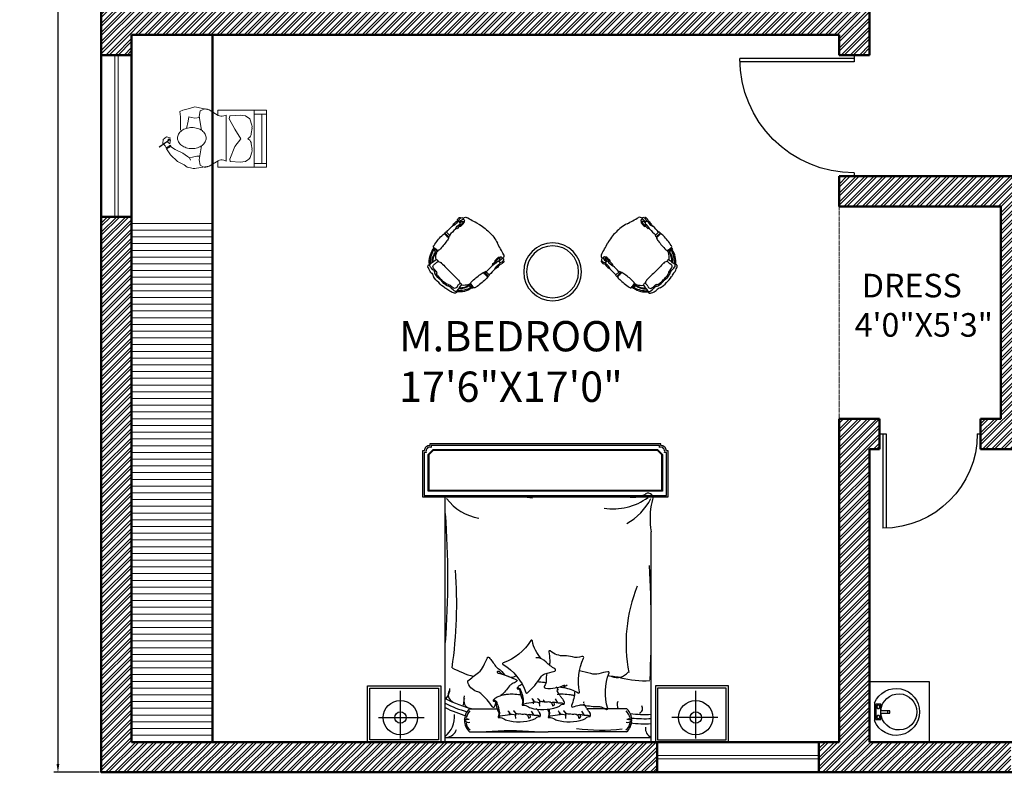
# Model space of a CAD drawing. Units: inches. Extents: x 3590 to 5167, y 65 to 1917.
# Tile 26 of 100: x 4396 to 4688, y 1326 to 1549. Entities that reach past the tile are written whole.
import ezdxf

# ---------------------------------------------------------------- set-up
doc = ezdxf.new("R2010")
doc.units = ezdxf.units.IN
doc.linetypes.add('DASHED', pattern=[0.75, 0.5, -0.25])
for name, color, linetype, lineweight in [('A-ANNO-DIMS', 2, 'Continuous', 18), ('A-AREA-IDEN', 7, 'Continuous', 18), ('A-DOOR', 3, 'Continuous', 25), ('A-FLOR-FIXT', 8, 'Continuous', 18), ('A-FURN', 21, 'Continuous', 18), ('A-GLAZ', 4, 'Continuous', 18), ('A-WALL', 7, 'Continuous', 50), ('A-WALL-PATT', 251, 'Continuous', 13), ('S-BEAM-OVHD', 7, 'DASHED', 18)]:
    doc.layers.add(name, color=color, linetype=linetype, lineweight=lineweight)
for name, color, linetype in [('FUR', 42, 'Continuous'), ('furn', 7, 'Continuous'), ('HA-FUR', 8, 'Continuous'), ('HA-P', 8, 'Continuous'), ('SAN', 5, 'Continuous'), ('SANTEH', 7, 'Continuous'), ('wood', 26, 'Continuous')]:
    doc.layers.add(name, color=color, linetype=linetype)
doc.styles.get("Standard").update_dxf_attribs({"font": 'arial.ttf'})
doc.dimstyles.new('ISO-25', dxfattribs={"dimtxt": 9, "dimasz": 2.5, "dimexe": 1.25, "dimexo": 0.625, "dimtad": 1, "dimdec": 1, "dimlunit": 3, "dimtxsty": 'Standard', "dimcen": 2.5, "dimadec": 0, "dimazin": 0, "dimtfac": 1, "dimtdec": 1, "dimtmove": 0, "dimatfit": 3, "dimfxl": 1, "dimarcsym": 0})

# ---------------------------------------------------------------- blocks, each defined once
blk = doc.blocks.new('*D102')
at = {"layer": 'A-ANNO-DIMS', "color": 0, "lineweight": -2, "transparency": 16777216}
for p, q in [((4419.65, 1806), (4406.15, 1806)), ((4407.4, 1803.5), (4407.4, 1328.5)), ((4419.65, 1326), (4406.15, 1326))]:
    blk.add_line(p, q, dxfattribs=at)
at = {"layer": 'A-ANNO-DIMS', "color": 0, "transparency": 16777216}
for points in [[(4406.98, 1803.5), (4407.82, 1803.5), (4407.4, 1806)], [(4406.98, 1328.5), (4407.82, 1328.5), (4407.4, 1326)]]:
    blk.add_solid(points, dxfattribs=at)
at = {"layer": 'Defpoints', "color": 0, "transparency": 16777216}
for p in [(4420.27, 1806), (4407.4, 1326), (4420.27, 1326)]:
    blk.add_point(p, dxfattribs=at)
at = {"layer": 'A-ANNO-DIMS', "color": 0, "transparency": 16777216, "insert": (4402.18, 1566), "char_height": 9, "attachment_point": 5, "rotation": 90}
blk.add_mtext("40'", dxfattribs=at)
blk = doc.blocks.new('D2')
for p, q in [((1, 0), (1, 28)), ((2, 0), (2, 27.98)), ((0, 0), (2, 0)), ((29, 0), (30, 0))]:
    blk.add_line(p, q)
at = {"ltscale": 0.5}
blk.add_arc((1, 0), 28, 0, 90, dxfattribs=at)
blk = doc.blocks.new('D1')
for p, q in [((1, 0), (1, 34)), ((2, 0), (2, 33.99)), ((0, 0), (2, 0)), ((35, 0), (36, 0))]:
    blk.add_line(p, q)
at = {"ltscale": 0.5}
blk.add_arc((1, 0), 34, 0, 90, dxfattribs=at)
blk = doc.blocks.new('r11')
at = {"layer": 'SANTEH', "ltscale": 5}
for p, q in [((0, 0), (600, 0)), ((0, -600), (0, 0)), ((600, 0), (600, -600)), ((210.5, -50), (389.5, -50)), ((210.5, -50), (210.5, -50)), ((223.8, -63.2), (376.2, -63.2)), ((223.8, -113.2), (223.8, -63.2)), ((232.7, -78.7), (249.2, -69.1)), ((232.7, -97.7), (232.7, -78.7)), ((249.2, -107.2), (232.7, -97.7)), ((249.2, -69.1), (265.7, -78.7)), ((265.7, -97.7), (249.2, -107.2)), ((265.7, -78.7), (265.7, -97.7)), ((334.3, -78.7), (350.8, -69.1)), ((334.3, -97.7), (334.3, -78.7)), ((350.8, -107.2), (334.3, -97.7)), ((350.8, -69.1), (367.3, -78.7)), ((367.3, -97.7), (350.8, -107.2)), ((367.3, -78.7), (367.3, -97.7)), ((376.2, -63.2), (376.2, -113.2)), ((376.2, -113.2), (223.8, -113.2)), ((288, -201.6), (288, -113.2)), ((312, -184.3), (288, -184.3)), ((312, -113.2), (312, -201.6)), ((312, -201.6), (288, -201.6)), ((600, -600), (0, -600))]:
    blk.add_line(p, q, dxfattribs=at)
for centre, radius, start, end in [((300, -266.2), 234, 112.50001, 67.49999), ((300, -293), 180.2, 93.8183, 86.1817)]:
    blk.add_arc(centre, radius, start, end, dxfattribs=at)
blk = doc.blocks.new('A$C0A42580C')
at = {"layer": 'SAN'}
for p, q in [((0.2873, 0.0301), (0.2873, 0.4484)), ((2.8678, 0.0301), (2.8678, 0.4484)), ((0.0949, 0.2135), (0.4958, 0.2135)), ((3.0601, 0.2135), (2.6592, 0.2135))]:
    blk.add_line(p, q, dxfattribs=at)
for centre, radius in [((0.2873, 0.2135), 0.15), ((2.8678, 0.2135), 0.15), ((0.2873, 0.2135), 0.05), ((2.8678, 0.2135), 0.05)]:
    blk.add_circle(centre, radius, dxfattribs=at)
at = {"layer": 'wood'}
for p, q in [((0.6775, 0.8851), (0.6775, 2.1392)), ((2.4775, 0.8016), (2.4775, 1.838)), ((2.4775, 0), (2.4775, 0.8016)), ((1.6633, 0.3438), (1.6434, 0.3761)), ((0.888, 0.289), (1.1327, 0.289)), ((1.4538, 0.2362), (1.434, 0.2685)), ((1.5, 0.3423), (1.5016, 0.3142)), ((1.8919, 0.2362), (1.8721, 0.2685)), ((2.267, 0.289), (1.9163, 0.289)), ((1.2906, 0.2348), (1.2921, 0.2067)), ((1.7287, 0.2348), (1.7302, 0.2067)), ((0.8909, 0.089), (1.5775, 0.089)), ((2.2642, 0.089), (1.5775, 0.089)), ((0.6775, 0.039), (2.4775, 0.039)), ((0.6775, 0), (2.4775, 0))]:
    blk.add_line(p, q, dxfattribs=at)
blk.add_lwpolyline([(0.6775, 0), (0.6775, 0.8851)], dxfattribs=at)
for points in [[(1.516, 0.7294, -0.128392), (1.4401, 0.8834, 0.70791), (1.427, 0.8863, -0.16964), (1.1848, 0.6919, 0.664036), (1.184, 0.6776, -0.184649), (1.3819, 0.4332, 0.662242), (1.3969, 0.4309, 0.078539), (1.5137, 0.5669, -0.1736), (1.5484, 0.5947, -0.02159), (1.6357, 0.6205, 0.697276), (1.6379, 0.6405, -0.093019), (1.5606, 0.699, 0.216632), (1.4719, 0.7371, -2.511293)], [(1.6795, 0.4818, 0.263265), (1.7191, 0.4839, -0.026108), (1.743, 0.4973, 0.027613), (1.7137, 0.4764, -0.089259), (1.8403, 0.429, 0.662242), (1.8528, 0.4376, -0.162037), (1.8882, 0.732, 0.676499), (1.8733, 0.748, -0.160513), (1.7901, 0.7439, 0.07473), (1.7202, 0.7523, -0.187721), (1.5966, 0.7963, 0.70791), (1.5851, 0.7895, -0.010003), (1.5921, 0.7143, -0.07079), (1.5891, 0.6719, 0.099539)], [(1.1211, 0.3454, 0.032543), (1.1095, 0.3091, -0.658965), (1.0917, 0.3063, 0.074753), (0.9887, 0.4234, 0.100988), (0.953, 0.4429, -0.270711), (0.8753, 0.5273, -0.276825), (0.8775, 0.5337, -0.014937), (0.9701, 0.6081, 0.134834), (1.0135, 0.6643, -0.023706), (1.0474, 0.7372, -0.664036), (1.0616, 0.7394, -0.035987), (1.119, 0.6627, 0.118631), (1.1415, 0.6412, -0.132738), (1.1955, 0.5864)], [(1.1759, 0.5928, 0.013884), (1.1549, 0.6131, 0.174178), (1.1437, 0.6177, 0.104076), (1.1358, 0.6165, 0.389829), (1.1324, 0.6097, 0.296089), (1.1415, 0.6019, -0.036701), (1.1572, 0.5985, -0.040547), (1.3022, 0.543, -0.70791), (1.3021, 0.5296, -0.016811), (1.2631, 0.5085, 0.11866), (1.2414, 0.4904, -0.048791), (1.1649, 0.4055, 0.103757)], [(1.8113, 0.4446, -0.069098), (1.7831, 0.3187, 0.658965), (1.7961, 0.3062, -0.049789), (1.8516, 0.3234, -0.103757), (1.8905, 0.3233, 0.055725), (2.0203, 0.3103, -0.11866), (2.0478, 0.304, 0.016811), (2.0881, 0.2856, 0.70791), (2.0989, 0.2936, -0.16964), (2.1104, 0.604, 0.664036), (2.1001, 0.6139, 0.023706), (2.0214, 0.597, -0.134834), (1.9505, 0.5976, 0.012748), (1.8522, 0.6228)], [(1.5674, 0.601, 0.057807), (1.5606, 0.5339, -0.173425), (1.5457, 0.49, 0.589988), (1.5538, 0.4706, 0.137312), (1.7236, 0.4985, 0.137312)], [(1.3107, 0.4764, 0.145733), (1.3069, 0.4677, 0.488583), (1.3089, 0.4657, -0.012138), (1.3131, 0.4661, -0.125673), (1.3213, 0.4646, -0.750706)], [(1.3153, 0.4751, -0.274893), (1.3379, 0.4529, 0.051436), (1.3468, 0.4293, -0.086628), (1.3532, 0.4078, 0.040196), (1.3593, 0.3772, -0.184744), (1.3556, 0.3344, -2.554464)], [(1.317, 0.4683, -0.060098), (1.3283, 0.4571, -0.16247), (1.3313, 0.4487, 0.120018), (1.3493, 0.3815, -0.060072), (1.3541, 0.3695, -0.13107), (1.3541, 0.3395, -0.024415), (1.3534, 0.3373, 0.070398), (1.3503, 0.3233, 0.528689), (1.3524, 0.3216, -0.069388), (1.3557, 0.3222, -0.158233), (1.4075, 0.3065, 0.085461), (1.4255, 0.2981, 0.147196), (1.6571, 0.3041, 0.10985), (1.6823, 0.3191, -0.179095), (1.7126, 0.3319, -2.318897)], [(1.1013, 0.3688, 0.145733), (1.0975, 0.3601, 0.488583), (1.0995, 0.3581, -0.012138), (1.1036, 0.3585, -0.125673), (1.1119, 0.357, -0.750706)], [(1.1059, 0.3675, -0.274893), (1.1285, 0.3453, 0.051436), (1.1373, 0.3217, -0.086628), (1.1438, 0.3003, 0.040196), (1.1499, 0.2696, -0.184744), (1.1462, 0.2269, -2.554464)], [(1.1076, 0.3607, -0.060098), (1.1189, 0.3495, -0.16247), (1.1219, 0.3411, 0.120018), (1.1399, 0.2739, -0.060072), (1.1447, 0.2619, -0.13107), (1.1447, 0.2319, -0.024415), (1.144, 0.2297, 0.070398), (1.1409, 0.2157, 0.528689), (1.143, 0.2141, -0.069388), (1.1463, 0.2146, -0.158233), (1.1981, 0.1989, 0.085461), (1.2161, 0.1905, 0.147196), (1.4477, 0.1965, 0.10985), (1.4728, 0.2115, -0.179095), (1.5032, 0.2244, -2.318897)], [(1.3509, 0.3219, -0.117141), (1.3688, 0.335, -0.025084), (1.4533, 0.348, 0.033691)], [(1.4359, 0.3803, -0.198519), (1.452, 0.3494, 0.826402), (1.4558, 0.349, 0.095956), (1.4561, 0.3528, 0.242899), (1.4461, 0.3686, -17.523452)], [(1.5447, 0.3525, -0.083557), (1.507, 0.3546, 0.203162), (1.4851, 0.3792, -0.208037), (1.5043, 0.3409, 0.124669), (1.4432, 0.3469, 0.965934)], [(1.5394, 0.3688, 0.145733), (1.5356, 0.3601, 0.488583), (1.5376, 0.3581, -0.012138), (1.5418, 0.3585, -0.125673), (1.55, 0.357, -0.750706)], [(1.5447, 0.3525, -0.008229), (1.5728, 0.3519, 0.033691)], [(1.5728, 0.3519, -0.46905), (1.6152, 0.321, 0.420988), (1.62, 0.3169, 0.857652), (1.6221, 0.3484, 0.548526)], [(1.603, 0.3451, -0.099719), (1.6221, 0.3484, 0.102691)], [(1.6214, 0.3487, -0.010168), (1.6558, 0.3447, 0.033691), (1.6907, 0.3423, -0.220869), (1.7148, 0.3311, -0.288972)], [(1.2265, 0.2728, -0.198519), (1.2426, 0.2418, 0.826402), (1.2463, 0.2415, 0.095956), (1.2467, 0.2452, 0.242899), (1.2366, 0.2611, -17.523452)], [(1.3353, 0.2449, -0.083557), (1.2976, 0.247, 0.203162), (1.2757, 0.2717, -0.208037), (1.2948, 0.2333, 0.124669), (1.2338, 0.2393, 0.965934)], [(1.5721, 0.286, 0.022869), (1.578, 0.2739, -0.060072), (1.5828, 0.2619, -0.13107), (1.5828, 0.2319, -0.024415), (1.5821, 0.2297, 0.070398), (1.579, 0.2157, 0.528689), (1.5811, 0.2141, -0.069388), (1.5844, 0.2146, -0.158233), (1.6362, 0.1989, 0.085461), (1.6542, 0.1905, 0.147196), (1.8858, 0.1965, 0.10985), (1.911, 0.2115, -0.179095), (1.9413, 0.2244, -2.318897)], [(1.5838, 0.2873, 0.023398), (1.588, 0.2696, -0.184744), (1.5843, 0.2269, -2.554464)], [(1.6646, 0.2728, -0.198519), (1.6807, 0.2418, 0.826402), (1.6845, 0.2415, 0.095956), (1.6848, 0.2452, 0.242899), (1.6748, 0.2611, -17.523452)], [(1.7734, 0.2449, -0.083557), (1.7357, 0.247, 0.203162), (1.7138, 0.2717, -0.208037), (1.733, 0.2333, 0.124669), (1.6719, 0.2393, 0.965934)], [(1.1415, 0.2143, -0.117141), (1.1594, 0.2274, -0.025084), (1.2439, 0.2405, 0.033691)], [(1.3353, 0.2449, -0.008229), (1.3633, 0.2443, 0.033691)], [(1.3633, 0.2443, -0.46905), (1.4058, 0.2134, 0.420988), (1.4106, 0.2093, 0.857652), (1.4127, 0.2408, 0.548526)], [(1.3936, 0.2375, -0.099719), (1.4127, 0.2408, 0.102691)], [(1.412, 0.2411, -0.010168), (1.4464, 0.2371, 0.033691), (1.4812, 0.2348, -0.220869), (1.5054, 0.2235, -0.288972)], [(1.5796, 0.2143, -0.117141), (1.5975, 0.2274, -0.025084), (1.682, 0.2405, 0.033691)], [(1.7734, 0.2449, -0.008229), (1.8015, 0.2443, 0.033691)], [(1.8015, 0.2443, -0.46905), (1.8439, 0.2134, 0.420988), (1.8487, 0.2093, 0.857652), (1.8508, 0.2408, 0.548526)], [(1.8317, 0.2375, -0.099719), (1.8508, 0.2408, 0.102691)], [(1.8501, 0.2411, -0.010168), (1.8845, 0.2371, 0.033691), (1.9193, 0.2348, -0.220869), (1.9435, 0.2235, -0.288972)]]:
    blk.add_lwpolyline(points, format="xyb", dxfattribs=at)
for points in [[(0.64, 0), (0, 0), (0, 0.49), (0.64, 0.49)], [(0.62, 0.02), (0.02, 0.02), (0.02, 0.47), (0.62, 0.47)], [(2.515, 0), (3.155, 0), (3.155, 0.49), (2.515, 0.49)], [(2.535, 0.02), (3.135, 0.02), (3.135, 0.47), (2.535, 0.47)]]:
    blk.add_lwpolyline(points, close=True, dxfattribs=at)
for centre, radius, start, end in [((1.0344, -2.14), 4.292, 84.56078, 94.7164), ((2.3125, 2.3833), 0.2443, 254.1515, 300.95574), ((2.4501, 2.1309), 0.0445, 324.18954, 118.92203), ((1.0494, 2.4026), 0.4515, 217.47941, 260.35986), ((2.0208, -11.0786), 13.2288, 88.75549, 92.51133), ((2.1491, 2.5471), 0.5083, 260.65485, 306.44155), ((2.0168, 2.3573), 0.5127, 299.08175, 333.44367), ((3.1371, 1.9502), 0.669, 166.6404, 189.65708), ((-7.0839, 1.4328), 7.7858, 355.84817, 4.15183), ((-3.167, 1.2143), 3.9465, 351.77286, 4.18386), ((-7.2439, 0.9937), 9.7233, 357.34474, 3.23068), ((3.5803, 0.8622), 1.3213, 157.81295, 191.15154), ((1.1611, 1.4181), 0.8768, 241.21362, 254.41879), ((2.181, 0.6859), 0.1221, 247.37754, 321.13165), ((1.2583, 0.6364), 0.0695, 238.58923, 301.92671), ((1.4714, 0.0722), 0.4528, 80.62397, 88.74059), ((1.4035, -0.3388), 0.8693, 79.71489, 80.62397), ((1.7861, -2.1601), 2.7557, 80.89877, 83.46656), ((2.4192, 1.3819), 0.8461, 255.77539, 273.25587), ((0.5904, 0.4689), 0.13, 317.38218, 359.70393), ((0.7723, 0.4131), 0.0674, 147.68233, 245.79865), ((1.3546, 0.4469), 0.0529, 114.21284, 146.15395), ((2.6126, -2.3504), 3.1201, 113.83178, 114.21284), ((1.6301, 0.4539), 0.0342, 31.14095, 54.95422), ((1.6709, 0.4489), 0.0156, 131.9623, 212.08127), ((1.6729, 0.4422), 0.0178, 140.41793, 157.63267), ((1.7235, 0.4818), 0.0777, 212.08127, 227.364), ((1.6635, 0.4499), 0.00568, 95.52245, 140.41793), ((1.5664, 0.4154), 0.1086, 24.20989, 31.14095), ((1.6627, 0.4587), 0.00309, 275.52245, 24.20989), ((1.1611, 1.3191), 1.0568, 242.76671, 257.10398), ((0.0312, 0.4583), 0.8174, 350.42368, 356.2506), ((0.9021, 0.3562), 0.0605, 155.8342, 254.41058), ((1.1452, 0.3394), 0.0529, 114.21284, 146.15395), ((2.4032, -2.458), 3.1201, 113.55686, 114.21284), ((1.2046, 0.2912), 0.121, 99.42032, 113.55686), ((1.2774, -0.1478), 0.5659, 95.90379, 99.42032), ((1.2626, -0.005), 0.4223, 88.74059, 95.90379), ((1.2619, -0.0354), 0.4528, 80.62397, 88.74059), ((1.1941, -0.4464), 0.8693, 79.45871, 80.62397), ((1.4207, 0.3463), 0.0342, 31.14095, 54.95422), ((1.4614, 0.3413), 0.0156, 131.9623, 212.08127), ((1.4635, 0.3347), 0.0178, 140.41793, 157.63267), ((1.4541, 0.3424), 0.00568, 95.52245, 140.41793), ((1.357, 0.3078), 0.1086, 24.20989, 31.14095), ((1.4533, 0.3511), 0.00309, 275.52245, 24.20989), ((1.7007, -0.005), 0.4223, 88.74059, 95.90379), ((1.6391, 0.3902), 0.0469, 17.32618, 47.364), ((1.7106, 0.4125), 0.028, 197.32618, 226.17302), ((1.6431, 0.3422), 0.0695, 26.61764, 46.17302), ((1.8202, 0.431), 0.1287, 206.61764, 215.96192), ((1.7001, -0.0354), 0.4528, 80.62397, 88.74059), ((1.6975, 0.3419), 0.023, 350.76434, 35.96192), ((1.6322, -0.4464), 0.8693, 78.43923, 80.62397), ((1.9016, 0.3347), 0.0178, 140.41793, 157.63267), ((1.8922, 0.3424), 0.00568, 95.52245, 140.41793), ((2.2511, 0.3256), 0.071, 155.86842, 211.04513), ((1.1611, 1.3191), 1.0937, 243.75553, 254.4906), ((1.1611, 1.2816), 1.0937, 243.75553, 254.38927), ((0.9846, 0.1903), 0.1381, 134.39284, 227.23745), ((0.9986, 0.1735), 0.1427, 136.58239, 164.9725), ((1.5012, 0.305), 0.028, 197.32618, 226.17302), ((1.4337, 0.2347), 0.0695, 26.61764, 46.17302), ((1.6108, 0.3235), 0.1287, 206.61764, 215.96192), ((1.715, 0.3349), 0.00379, 207.1817, 328.02977), ((1.7058, 0.3406), 0.0145, 328.02977, 350.76434), ((1.9522, 0.3743), 0.0777, 212.08127, 227.364), ((1.8678, 0.2827), 0.0469, 17.32618, 47.364), ((1.9393, 0.305), 0.028, 197.32618, 226.17302), ((1.8718, 0.2347), 0.0695, 26.61764, 46.17302), ((2.0489, 0.3235), 0.1287, 206.61764, 215.96192), ((2.1565, 0.1735), 0.1427, 15.0275, 43.41761), ((2.1704, 0.1903), 0.1381, 312.76255, 45.60716), ((2.3616, 0.2915), 0.0419, 290.78583, 35.36309), ((0.5293, 0.2241), 0.2307, 309.63048, 4.27465), ((0.8396, 0.185), 0.0112, 314.89662, 45.10338), ((0.8413, 0.1846), 0.0128, 299.47062, 57.44416), ((0.8844, 0.2286), 0.0569, 229.70587, 281.11527), ((0.8802, 0.1371), 0.0592, 81.47786, 123.11925), ((0.8698, 0.1793), 0.0229, 77.14902, 159.1786), ((1.5055, 0.2273), 0.00379, 207.1817, 328.02977), ((1.4881, 0.2344), 0.023, 350.76434, 35.96192), ((1.4964, 0.233), 0.0145, 328.02977, 350.76434), ((1.9436, 0.2273), 0.00379, 207.1817, 328.02977), ((1.9262, 0.2344), 0.023, 350.76434, 35.96192), ((1.9345, 0.233), 0.0145, 328.02977, 350.76434), ((2.2706, 0.2286), 0.0569, 258.88473, 310.29413), ((2.2749, 0.1371), 0.0592, 56.88075, 98.52214), ((2.2853, 0.1793), 0.0229, 20.8214, 102.85098), ((2.4192, 1.2667), 1.0261, 263.09035, 273.25587), ((2.3138, 0.1846), 0.0128, 122.55584, 240.52938), ((2.3154, 0.185), 0.0112, 134.89662, 225.10338), ((2.4192, 1.2667), 1.0629, 263.94374, 273.25587), ((0.6729, 0.151), 0.1135, 279.23824, 338.73819), ((0.9466, 0.1765), 0.0862, 185.53723, 234.68694), ((1.2481, -2.5919), 2.6893, 85.4722, 94.5278), ((2.0447, 1.7022), 1.5979, 262.13639, 276.48786), ((2.2085, 0.1765), 0.0862, 305.31306, 354.46277), ((2.4192, 1.2218), 1.0629, 263.23622, 273.25587), ((2.508, 0.1152), 0.0792, 169.94668, 248.24015)]:
    blk.add_arc(centre, radius, start, end, dxfattribs=at)
blk = doc.blocks.new('A$C623F1DA0')
at = {"layer": 'FUR'}
blk.add_lwpolyline([(0.628, 2.912, 0.414214), (0.562, 2.978), (0.562, 3), (0, 3), (0, 0), (0.562, 0), (0.562, 0.022, 0.414214), (0.628, 0.088), (0.65, 0.088), (0.65, 2.912)], format="xyb", close=True, dxfattribs=at)
at = {"layer": 'HA-FUR'}
blk.add_lwpolyline([(0.603, 2.892, 0.710288), (0.542, 2.953), (0.542, 2.98), (0.02, 2.98), (0.02, 0.02), (0.542, 0.02), (0.542, 0.047, 0.710288), (0.603, 0.108), (0.63, 0.108), (0.63, 2.892)], format="xyb", close=True, dxfattribs=at)
at = {"layer": 'HA-P'}
for points in [[(0.07, 2.93), (0.521, 2.93), (0.58, 2.871), (0.58, 0.129), (0.521, 0.07), (0.07, 0.07)], [(0.08, 2.92), (0.517, 2.92), (0.57, 2.867), (0.57, 0.133), (0.517, 0.08), (0.08, 0.08)]]:
    blk.add_lwpolyline(points, close=True, dxfattribs=at)
blk = doc.blocks.new('CHAIR6')
at = {"layer": 'furn'}
for p, q in [((0.41, 0.26), (0.409, 0.318)), ((0.428, 0.318), (0.427, 0.263)), ((0.41, -0.26), (0.409, -0.318)), ((0.428, -0.318), (0.427, -0.263))]:
    blk.add_line(p, q, dxfattribs=at)
for centre in [(0.405, 0.315), (0.405, 0.306), (0.217, 0.287), (0.219, 0.277), (0.22, 0.268), (0.221, 0.26), (0.222, 0.252), (0.223, 0.243), (0.405, 0.298), (0.405, 0.29), (0.406, 0.281), (0.405, 0.273), (0.406, 0.264), (0.217, -0.287), (0.219, -0.277), (0.22, -0.268), (0.221, -0.26), (0.222, -0.252), (0.223, -0.243), (0.406, -0.264), (0.405, -0.273), (0.406, -0.281), (0.405, -0.29), (0.405, -0.298), (0.405, -0.306), (0.405, -0.315)]:
    blk.add_circle(centre, 0.00425, dxfattribs=at)
for centre, radius, start, end in [((0.237, 0.291), 0.0162, 83.9773, 174.0092), ((0.372, -0.317), 0.638, 90.6066, 102.0554), ((0.377, 0.168), 0.153, 77.8964, 94.5268), ((3.364, 0.315), 2.963, 179.9011, 181.1479), ((0.418, 0.279), 0.04, 75.217, 102.1825), ((0.481, -0.309), 0.624, 87.1388, 94.8424), ((0.516, 0.348), 0.0344, 262.5365, 295.1239), ((0.554, 0.405), 0.1, 244.9615, 286.9262), ((0.557, 0.199), 0.121, 80.5687, 102.5802), ((0.569, 0.306), 0.0148, 11.9312, 56.7136), ((0.557, 0.368), 0.0592, 293.7073, 312.3115), ((0.581, 0.292), 0.0168, 1.9585, 81.7578), ((0.627, 0.253), 0.0606, 83.3314, 123.5905), ((0.615, 0.273), 0.0542, 72.7266, 108.7219), ((0.629, 0.318), 0.00734, 318.7265, 73.2046), ((0.633, 0.295), 0.0177, 352.6874, 85.2992), ((0.231, 0.078), 0.206, 99.5359, 142.9697), ((0.288, -0.009), 0.296, 107.467, 135.6907), ((0.22, 0.084), 0.164, 95.986, 137.8084), ((0.297, -0.027), 0.289, 108.9658, 130.7483), ((0.27, 0.102), 0.148, 115.7424, 145.5422), ((0.2, 0.33), 0.0425, 267.3788, 299.5385), ((0.508, 0.309), 0.31, 183.9213, 193.664), ((0.217, 0.209), 0.0298, 85.8824, 112.3894), ((0.91, 0.35), 0.7, 184.9582, 189.1744), ((0.204, 0.356), 0.119, 277.5474, 281.9349), ((2.236, 0.546), 2.032, 187.1641, 188.6742), ((0.243, 0.265), 0.029, 238.5377, 274.9353), ((0.251, 0.88), 0.644, 269.5737, 280.2481), ((0.357, 0.351), 0.106, 274.4213, 300.1481), ((0.412, 0.301), 0.0413, 267.6069, 291.9537), ((0.471, 1.044), 0.775, 266.7794, 273.3084), ((0.558, 0.149), 0.128, 78.3216, 109.437), ((0.517, 0.26), 0.0105, 7.9295, 98.404), ((0.548, 0.417), 0.157, 262.6911, 279.4279), ((0.576, 0.259), 0.00554, 151.0446, 320.6391), ((0.573, 0.254), 0.00119, 58.8883, 217.8317), ((0.586, 0.299), 0.0481, 252.1536, 277.044), ((0.575, 0.272), 0.00992, 261.0604, 17.0352), ((0.6, 0.611), 0.349, 266.3251, 275.7659), ((0.586, 0.259), 0.00592, 143.235, 315.8485), ((0.571, 0.299), 0.0282, 299.2631, 346.0553), ((0.54, 0.261), 0.0504, 352.1945, 0.4931), ((0.596, 0.265), 0.012, 240.9156, 292.3604), ((0.599, 0.223), 0.0286, 84.2359, 104.2257), ((0.621, 0.242), 0.0492, 62.0869, 124.0669), ((0.596, 0.232), 0.05, 38.3646, 93.2736), ((0.63, 0.259), 0.03, 175.2542, 190.1424), ((0.604, 0.261), 0.00773, 242.6807, 299.2264), ((0.605, 0.322), 0.0704, 267.2787, 279.3344), ((0.623, 0.26), 0.0167, 173.5024, 200.3975), ((0.61, 0.258), 0.0049, 236.8473, 330.7161), ((0.646, 0.262), 0.0322, 179.9162, 191.0366), ((0.618, 0.257), 0.00347, 207.2761, 12.1204), ((0.62, 0.264), 0.0117, 254.3857, 324.079), ((0.626, 0.265), 0.00881, 232.8615, 349.2883), ((0.71, 0.267), 0.0896, 182.9909, 185.7082), ((0.635, 0.276), 0.0126, 270.9628, 46.1593), ((0.624, 0.308), 0.0303, 309.8512, 329.8717), ((0.651, 0.258), 0.0349, 27.0208, 91.1191), ((5.591, 1.641), 5.096, 195.566, 197.1124), ((-0.099, 0.131), 0.116, 336.0762, 0.2883), ((0.175, 0.114), 0.159, 153.5859, 173.6765), ((0.057, 0.18), 0.0247, 65.1084, 167.8729), ((0.064, 0.08), 0.0277, 124.7421, 163.8327), ((0.009, 0.12), 0.0432, 336.8405, 13.1255), ((0.208, 0.139), 0.158, 161.7945, 183.4813), ((0.042, 0.101), 0.0209, 307.2671, 6.2804), ((0.076, 0.176), 0.0215, 90.4966, 146.0411), ((0.234, 0.103), 0.171, 161.3786, 179.7853), ((0.075, 0.206), 0.00875, 210.7256, 277.1225), ((0.096, 0.134), 0.0336, 65.79, 135.3719), ((1.294, 7.349), 7.255, 260.3299, 260.9616), ((0.132, 0.233), 0.0718, 252.5123, 277.4747), ((0.142, 0.148), 0.0139, 39.5976, 92.786), ((0.101, 0.175), 0.0542, 340.1354, 9.9737), ((0.112, 0.126), 0.0505, 352.8157, 37.4708), ((-4.033, 0.095), 4.196, 358.7024, 0.3415), ((0.344, 0.019), 0.396, 357.2491, 18.1081), ((0.24, 0.022), 0.241, 165.2285, 185.2845), ((0.27, 0.033), 0.239, 166.6572, 187.8069), ((0.458, 0.014), 0.416, 173.7493, 181.9752), ((0.09, 0.054), 0.0465, 139.2002, 173.5011), ((0.24, -0.022), 0.241, 174.7155, 194.7715), ((-0.099, -0.131), 0.116, 359.7117, 23.9238), ((0.27, -0.033), 0.239, 172.1931, 193.3428), ((0.064, -0.08), 0.0277, 196.1673, 235.2579), ((0.458, -0.014), 0.416, 178.0248, 186.2507), ((0.09, -0.054), 0.0465, 186.4989, 220.7998), ((0.042, -0.101), 0.0209, 353.7196, 52.7329), ((-4.033, -0.095), 4.196, 359.6585, 1.2976), ((0.344, -0.019), 0.396, 341.8919, 2.7509), ((0.175, -0.114), 0.159, 186.3235, 206.4141), ((0.057, -0.18), 0.0247, 192.1271, 294.8916), ((0.009, -0.12), 0.0432, 346.8745, 23.1595), ((0.208, -0.139), 0.158, 176.5187, 198.2055), ((0.076, -0.176), 0.0215, 213.9589, 269.5034), ((0.234, -0.103), 0.171, 180.2147, 198.6214), ((0.075, -0.206), 0.00875, 82.8775, 149.2744), ((0.231, -0.078), 0.206, 217.0303, 260.4641), ((0.096, -0.134), 0.0336, 224.6281, 294.21), ((1.294, -7.349), 7.255, 99.0384, 99.6701), ((0.288, 0.009), 0.296, 224.3093, 252.533), ((0.22, -0.084), 0.164, 222.1916, 264.014), ((0.297, 0.027), 0.289, 229.2517, 251.0342), ((0.132, -0.233), 0.0718, 82.5253, 107.4877), ((0.142, -0.148), 0.0139, 267.214, 320.4024), ((0.27, -0.102), 0.148, 214.4578, 244.2576), ((0.112, -0.126), 0.0505, 322.5292, 7.1843), ((0.101, -0.175), 0.0542, 350.0263, 19.8646), ((5.591, -1.641), 5.096, 162.8876, 164.434), ((0.508, -0.309), 0.31, 166.336, 176.0787), ((0.2, -0.33), 0.0425, 60.4615, 92.6212), ((0.217, -0.209), 0.0298, 247.6106, 274.1176), ((0.91, -0.35), 0.7, 170.8256, 175.0418), ((0.204, -0.356), 0.119, 78.0651, 82.4526), ((2.236, -0.546), 2.032, 171.3258, 172.8359), ((0.237, -0.291), 0.0162, 185.9908, 276.0227), ((0.243, -0.265), 0.029, 85.0647, 121.4623), ((0.251, -0.88), 0.644, 79.7519, 90.4263), ((0.357, -0.351), 0.106, 59.8519, 85.5787), ((3.364, -0.315), 2.963, 178.8521, 180.0989), ((0.412, -0.301), 0.0413, 68.0463, 92.3931), ((0.471, -1.044), 0.775, 86.6916, 93.2206), ((0.554, -0.405), 0.1, 73.0738, 115.0385), ((0.517, -0.26), 0.0105, 261.596, 352.0705), ((0.558, -0.149), 0.128, 250.563, 281.6784), ((0.548, -0.417), 0.157, 80.5721, 97.3089), ((0.573, -0.254), 0.00119, 142.1683, 301.1117), ((0.576, -0.259), 0.00554, 39.3609, 208.9554), ((0.586, -0.299), 0.0481, 82.956, 107.8464), ((0.575, -0.272), 0.00992, 342.9648, 98.9396), ((0.6, -0.611), 0.349, 84.2341, 93.6749), ((0.586, -0.259), 0.00592, 44.1515, 216.765), ((0.581, -0.292), 0.0168, 278.2422, 358.0415), ((0.571, -0.299), 0.0282, 13.9447, 60.7369), ((0.596, -0.265), 0.012, 67.6396, 119.0844), ((0.54, -0.261), 0.0504, 359.5069, 7.8055), ((0.599, -0.223), 0.0286, 255.7743, 275.7641), ((0.596, -0.232), 0.05, 266.7264, 321.6354), ((0.621, -0.242), 0.0492, 235.9331, 297.9131), ((0.627, -0.253), 0.0606, 236.4095, 276.6686), ((0.604, -0.261), 0.00773, 60.7736, 117.3193), ((0.63, -0.259), 0.03, 169.8576, 184.7458), ((0.605, -0.322), 0.0704, 80.6656, 92.7213), ((0.623, -0.26), 0.0167, 159.6025, 186.4976), ((0.61, -0.258), 0.0049, 29.2839, 123.1527), ((0.646, -0.262), 0.0322, 168.9634, 180.0838), ((0.618, -0.257), 0.00347, 347.8796, 152.7239), ((0.62, -0.264), 0.0117, 35.921, 105.6143), ((0.626, -0.265), 0.00881, 10.7117, 127.1385), ((0.71, -0.267), 0.0896, 174.2918, 177.0091), ((0.633, -0.295), 0.0177, 274.7008, 7.3126), ((0.635, -0.276), 0.0126, 313.8407, 89.0372), ((0.624, -0.308), 0.0303, 30.1283, 50.1488), ((0.651, -0.258), 0.0349, 268.8809, 332.9792), ((0.372, 0.317), 0.638, 257.9446, 269.3934), ((0.377, -0.168), 0.153, 265.4732, 282.1036), ((0.418, -0.279), 0.04, 257.8175, 284.783), ((0.481, 0.309), 0.624, 265.1576, 272.8612), ((0.516, -0.348), 0.0344, 64.8761, 97.4635), ((0.557, -0.199), 0.121, 257.4198, 279.4313), ((0.569, -0.306), 0.0148, 303.2864, 348.0688), ((0.557, -0.368), 0.0592, 47.6885, 66.2927), ((0.615, -0.273), 0.0542, 251.2781, 287.2734), ((0.629, -0.318), 0.00734, 286.7954, 41.2735)]:
    blk.add_arc(centre, radius, start, end, dxfattribs=at)
blk = doc.blocks.new('A$C78847651')
at = {"layer": 'furn'}
for radius in [0.3, 0.27]:
    blk.add_circle((1.292, 0.566), radius, dxfattribs=at)
at = {"layer": 'furn', "rotation": 315}
blk.add_blockref('CHAIR6', (0.11, 0.677), dxfattribs=at)
at = {"layer": 'furn', "xscale": -1, "rotation": 44.99999999999991}
blk.add_blockref('CHAIR6', (2.474, 0.677), dxfattribs=at)
blk = doc.blocks.new('DESK-CHAIR')
for p, q in [((3675.51, 1522.74), (3674.9, 1522.4)), ((3680.2, 1521.08), (3677.49, 1522.71)), ((3674.9, 1522.4), (3674.54, 1520.79)), ((3674.54, 1520.79), (3675.25, 1516.67)), ((3694.59, 1522.58), (3680.09, 1522.58)), ((3680.09, 1522.58), (3680.09, 1521.15)), ((3682.6, 1521.15), (3681.85, 1520.9)), ((3682.6, 1521.15), (3682.6, 1507.53)), ((3682.6, 1507.53), (3682.6, 1521.15)), ((3683.49, 1520.07), (3683.66, 1520.91)), ((3685.1, 1517.02), (3683.49, 1520.07)), ((3683.73, 1520.97), (3686.72, 1521.15)), ((3686.72, 1521.15), (3688.33, 1520.97)), ((3688.33, 1520.97), (3689.58, 1520.07)), ((3689.58, 1520.07), (3690.17, 1518.15)), ((3694.59, 1505.74), (3694.59, 1522.58)), ((3686.89, 1514.16), (3685.1, 1517.02)), ((3690.24, 1517.32), (3690.04, 1515.67)), ((3685.1, 1511.83), (3686.89, 1514.16)), ((3689.31, 1514.37), (3689.04, 1514.16)), ((3689.31, 1513.95), (3689.04, 1514.16)), ((3664.74, 1511.43), (3666.04, 1512.26)), ((3665.07, 1511.29), (3664.74, 1511.43)), ((3664.84, 1511.19), (3666.07, 1511.86)), ((3666.04, 1509.36), (3664.84, 1511.19)), ((3666.04, 1512.26), (3666.24, 1511.79)), ((3666.07, 1511.86), (3667.43, 1510.93)), ((3667.43, 1510.93), (3669.7, 1509.83)), ((3674.54, 1507.89), (3675.25, 1512.01)), ((3683.67, 1508.07), (3685.1, 1511.83)), ((3690.24, 1511), (3690.04, 1512.64)), ((3668.13, 1507.37), (3666.04, 1509.36)), ((3669.7, 1509.83), (3671.06, 1508.9)), ((3671.06, 1508.9), (3671.66, 1508.47)), ((3671.66, 1508.47), (3671.96, 1507.77)), ((3683.8, 1507.4), (3683.67, 1508.07)), ((3689.78, 1508.89), (3690.17, 1510.17)), ((3670.06, 1506.4), (3668.13, 1507.37)), ((3677.49, 1505.97), (3673.14, 1505.31)), ((3674.9, 1506.27), (3674.54, 1507.89)), ((3675.51, 1505.94), (3674.9, 1506.27)), ((3680.2, 1507.6), (3677.49, 1505.97)), ((3680.09, 1507.53), (3680.09, 1505.74)), ((3680.09, 1505.74), (3694.59, 1505.74)), ((3682.6, 1507.53), (3681.85, 1507.78)), ((3683.88, 1507.34), (3686.72, 1507.17)), ((3686.72, 1507.17), (3688.33, 1507.35)), ((3688.33, 1507.35), (3689.03, 1507.86))]:
    blk.add_line(p, q)
for points in [[(3677.49, 1522.71), (3673.28, 1523.65), (3671.67, 1523.12), (3669.7, 1522.58), (3668.81, 1522.22), (3668.99, 1520.61), (3668.99, 1519), (3668.99, 1516.67)], [(3664.74, 1511.43), (3664.42, 1512.05), (3663.77, 1512.78), (3663.87, 1513.9), (3664.88, 1514.67), (3665.92, 1514.37), (3665.9, 1514.02), (3665.32, 1514.02), (3665.3, 1513.1), (3665.82, 1512.66), (3666.07, 1513.84)], [(3671.66, 1508.47), (3672.6, 1508.69), (3673.82, 1508.93), (3674.7, 1508.93)], [(3670.06, 1506.4), (3671.04, 1505.75), (3672.02, 1505.46), (3672.8, 1505.31), (3673.24, 1505.31)]]:
    blk.add_lwpolyline(points)
at = {"const_width": 0.39}
blk.add_lwpolyline([(3666.01, 1513.98), (3662.61, 1511.61)], dxfattribs=at)
for centre, radius, start, end in [((3676.47, 1521), 1.98, 59.0235, 119.0669), ((3681.22, 1522.78), 1.98, 239.0235, 288.4436), ((3683.74, 1520.89), 0.0779, 93.3682, 168.6956), ((3683.74, 1520.89), 0.0779, 93.3682, 168.6956), ((3688.27, 1517.56), 1.98, 352.8785, 17.0946), ((3688.07, 1515.92), 1.98, 308.6739, 352.8785), ((3688.07, 1512.4), 1.98, 7.1215, 51.3261), ((3688.27, 1510.75), 1.98, 342.9054, 7.1215), ((3687.88, 1509.47), 1.98, 305.5514, 342.9054), ((3676.47, 1507.67), 1.98, 240.9331, 300.9765), ((3681.22, 1505.89), 1.98, 71.5564, 120.9765), ((3683.88, 1507.42), 0.0779, 191.3044, 266.6318)]:
    blk.add_arc(centre, radius, start, end)

msp = doc.modelspace()

# ---------------------------------------------------------------- hatches: boundary and pattern name
at = {"layer": 'A-WALL-PATT', "transparency": 33554687}
h = msp.add_hatch(dxfattribs=at)
h.set_pattern_fill('ANSI32', color=256, scale=0.2)
h.paths.add_polyline_path([(4684.27, 1806), (4591.27, 1806), (4591.27, 1797), (4639.27, 1797), (4639.27, 1791), (4648.27, 1791), (4648.27, 1797), (4684.27, 1797)])
h.paths.add_polyline_path([(4543.27, 1806), (4420.27, 1806), (4420.27, 1785), (4429.27, 1785), (4429.27, 1797), (4445.92, 1797), (4543.27, 1797)])
h.paths.add_polyline_path([(4828.27, 1806), (4744.27, 1806), (4744.27, 1797), (4828.27, 1797)])
h.paths.add_polyline_path([(4648.27, 1755), (4639.27, 1755), (4639.27, 1656), (4546.27, 1656), (4546.27, 1650), (4549.27, 1650), (4549.27, 1554), (4429.27, 1554), (4429.27, 1584), (4420.27, 1584), (4420.27, 1539), (4429.27, 1539), (4429.27, 1545), (4639.27, 1545), (4639.27, 1539), (4648.27, 1539), (4648.27, 1560), (4639.27, 1560), (4639.27, 1554), (4555.27, 1554), (4555.27, 1650), (4639.27, 1650), (4639.27, 1590), (4648.27, 1590)])
h.paths.add_polyline_path([(4516.27, 1656), (4429.27, 1656), (4429.27, 1737), (4420.27, 1737), (4420.27, 1620), (4429.27, 1620), (4429.27, 1650), (4516.27, 1650)], flags=17)
h.paths.add_polyline_path([(5080.27, 1806), (4888.27, 1806), (4888.27, 1797), (4924.27, 1797), (4924.27, 1755), (4933.27, 1755), (4933.27, 1797), (5071.27, 1797), (5071.27, 1335), (4933.27, 1335), (4933.27, 1566), (4924.27, 1566), (4924.27, 1335), (4898.77, 1335), (4898.77, 1326), (5080.27, 1326)])
h.paths.add_polyline_path([(4933.27, 1719), (4924.27, 1719), (4924.27, 1638), (4933.27, 1638)], flags=17)
h.paths.add_polyline_path([(4802.77, 1335), (4777.27, 1335), (4777.27, 1503), (4756.27, 1503), (4756.27, 1494), (4768.27, 1494), (4768.27, 1431), (4696.27, 1431), (4696.27, 1494), (4708.27, 1494), (4708.27, 1503), (4639.27, 1503), (4639.27, 1494), (4687.27, 1494), (4687.27, 1431), (4681.27, 1431), (4681.27, 1422), (4768.27, 1422), (4768.27, 1335), (4726.27, 1335), (4726.27, 1326), (4802.77, 1326)])
h.paths.add_polyline_path([(4690.27, 1335), (4648.27, 1335), (4648.27, 1352.87), (4648.27, 1422), (4651.27, 1422), (4651.27, 1431), (4639.27, 1431), (4639.27, 1335), (4633.27, 1335), (4633.27, 1326), (4690.27, 1326)])
h.paths.add_polyline_path([(4585.27, 1335), (4584.72, 1335), (4429.27, 1335), (4429.27, 1491), (4420.27, 1491), (4420.27, 1326), (4585.27, 1326)])

# ---------------------------------------------------------------- linework, layer by layer
at = {"layer": 'A-FURN'}
for p, q in [((4465.6, 1505.74), (4465.6, 1522.58)), ((4465.6, 1521.43), (4469.36, 1521.43)), ((4467.92, 1506.84), (4467.92, 1521.43)), ((4465.6, 1506.84), (4469.36, 1506.84)), ((4453.27, 1489), (4429.27, 1489)), ((4453.27, 1487), (4429.27, 1487)), ((4453.27, 1485), (4429.27, 1485)), ((4453.27, 1483), (4429.27, 1483)), ((4453.27, 1481), (4429.27, 1481)), ((4453.27, 1479), (4429.27, 1479)), ((4453.27, 1477), (4429.27, 1477)), ((4453.27, 1475), (4429.27, 1475)), ((4453.27, 1473), (4429.27, 1473)), ((4453.27, 1471), (4429.27, 1471)), ((4453.27, 1469), (4429.27, 1469)), ((4453.27, 1467), (4429.27, 1467)), ((4453.27, 1465), (4429.27, 1465)), ((4453.27, 1463), (4429.27, 1463)), ((4453.27, 1461), (4429.27, 1461)), ((4453.27, 1459), (4429.27, 1459)), ((4453.27, 1457), (4429.27, 1457)), ((4453.27, 1455), (4429.27, 1455)), ((4453.27, 1453), (4429.27, 1453)), ((4453.27, 1451), (4429.27, 1451)), ((4453.27, 1449), (4429.27, 1449)), ((4453.27, 1447), (4429.27, 1447)), ((4453.27, 1445), (4429.27, 1445)), ((4453.27, 1443), (4429.27, 1443)), ((4453.27, 1441), (4429.27, 1441)), ((4453.27, 1439), (4429.27, 1439)), ((4453.27, 1437), (4429.27, 1437)), ((4453.27, 1435), (4429.27, 1435)), ((4453.27, 1433), (4429.27, 1433)), ((4453.27, 1431), (4429.27, 1431)), ((4453.27, 1429), (4429.27, 1429)), ((4453.27, 1427), (4429.27, 1427)), ((4453.27, 1425), (4429.27, 1425)), ((4453.27, 1423), (4429.27, 1423)), ((4453.27, 1421), (4429.27, 1421)), ((4453.27, 1419), (4429.27, 1419)), ((4453.27, 1417), (4429.27, 1417)), ((4453.27, 1415), (4429.27, 1415)), ((4453.27, 1413), (4429.27, 1413)), ((4453.27, 1411), (4429.27, 1411)), ((4453.27, 1409), (4429.27, 1409)), ((4453.27, 1407), (4429.27, 1407)), ((4453.27, 1405), (4429.27, 1405)), ((4453.27, 1403), (4429.27, 1403)), ((4453.27, 1401), (4429.27, 1401)), ((4453.27, 1399), (4429.27, 1399)), ((4453.27, 1397), (4429.27, 1397)), ((4453.27, 1395), (4429.27, 1395)), ((4453.27, 1393), (4429.27, 1393)), ((4453.27, 1391), (4429.27, 1391)), ((4453.27, 1389), (4429.27, 1389)), ((4453.27, 1387), (4429.27, 1387)), ((4453.27, 1385), (4429.27, 1385)), ((4453.27, 1383), (4429.27, 1383)), ((4453.27, 1381), (4429.27, 1381)), ((4453.27, 1379), (4429.27, 1379)), ((4453.27, 1377), (4429.27, 1377)), ((4453.27, 1375), (4429.27, 1375)), ((4453.27, 1373), (4429.27, 1373)), ((4453.27, 1371), (4429.27, 1371)), ((4453.27, 1369), (4429.27, 1369)), ((4453.27, 1367), (4429.27, 1367)), ((4453.27, 1365), (4429.27, 1365)), ((4453.27, 1363), (4429.27, 1363)), ((4453.27, 1361), (4429.27, 1361)), ((4453.27, 1359), (4429.27, 1359)), ((4453.27, 1357), (4429.27, 1357)), ((4453.27, 1355), (4429.27, 1355)), ((4453.27, 1353), (4429.27, 1353)), ((4453.27, 1351), (4429.27, 1351)), ((4453.27, 1349), (4429.27, 1349)), ((4453.27, 1347), (4429.27, 1347)), ((4453.27, 1345), (4429.27, 1345)), ((4453.27, 1343), (4429.27, 1343)), ((4453.27, 1343), (4429.27, 1343)), ((4453.27, 1341), (4429.27, 1341)), ((4453.27, 1339), (4429.27, 1339)), ((4453.27, 1337), (4429.27, 1337))]:
    msp.add_line(p, q, dxfattribs=at)
msp.add_lwpolyline([(4445.54, 1517.2), (4446.08, 1519.35), (4446.26, 1520.61), (4448.05, 1520.25), (4449.48, 1520.43)], dxfattribs=at)
msp.add_lwpolyline([(4447.15, 1511.23, 0.07405), (4448.83, 1511.48, 0.084801), (4450.16, 1512.14, 0.106336), (4451.1, 1513.21, 0.128955), (4451.4, 1514.35, 0.128955), (4451.1, 1515.49, 0.106336), (4450.16, 1516.56, 0.084801), (4448.83, 1517.22, 0.07405), (4447.15, 1517.47, 0.07405), (4445.48, 1517.22, 0.084801), (4444.15, 1516.56, 0.106336), (4443.21, 1515.49, 0.128955), (4442.91, 1514.35, 0.128955), (4443.21, 1513.21, 0.106336), (4444.15, 1512.14, 0.084801), (4445.48, 1511.48, 0.07405)], format="xyb", close=True, dxfattribs=at)
at = {"layer": 'A-GLAZ'}
for p, q in [((4424.27, 1491), (4424.27, 1539)), ((4425.27, 1491), (4425.27, 1539)), ((4633.27, 1331), (4585.27, 1331)), ((4633.27, 1330), (4585.27, 1330))]:
    msp.add_line(p, q, dxfattribs=at)
at = {"layer": 'A-WALL'}
for p, q in [((4648.27, 1539), (4648.27, 1560)), ((4639.27, 1545), (4429.27, 1545)), ((4429.27, 1335), (4429.27, 1545)), ((4453.27, 1335), (4453.27, 1545)), ((4639.27, 1539), (4639.27, 1545)), ((4429.27, 1539), (4420.27, 1539)), ((4648.27, 1539), (4639.27, 1539)), ((4708.27, 1503), (4639.27, 1503)), ((4639.27, 1494), (4639.27, 1503)), ((4687.27, 1494), (4639.27, 1494)), ((4687.27, 1431), (4687.27, 1494)), ((4429.27, 1491), (4420.27, 1491)), ((4651.27, 1431), (4639.27, 1431)), ((4639.27, 1335), (4639.27, 1431)), ((4651.27, 1422), (4651.27, 1431)), ((4687.27, 1431), (4681.27, 1431)), ((4681.27, 1422), (4681.27, 1431)), ((4651.27, 1422), (4648.27, 1422)), ((4648.27, 1335), (4648.27, 1422)), ((4768.27, 1422), (4681.27, 1422)), ((4639.27, 1335), (4429.27, 1335)), ((4585.27, 1326), (4585.27, 1335)), ((4633.27, 1326), (4633.27, 1335)), ((4768.27, 1335), (4648.27, 1335))]:
    msp.add_line(p, q, dxfattribs=at)
msp.add_lwpolyline([(5080.27, 1806), (5080.27, 1326), (4420.27, 1326), (4420.27, 1806)], close=True, dxfattribs=at)
at = {"layer": 'S-BEAM-OVHD', "ltscale": 0.5}
msp.add_line((4639.27, 1494), (4639.27, 1431), dxfattribs=at)

# ---------------------------------------------------------------- block references
at = {"layer": 'A-DOOR', "xscale": -1}
for name, p, rotation in [('D1', (4643.77, 1539), 90), ('D2', (4651.27, 1426.5), 180)]:
    msp.add_blockref(name, p, dxfattribs=dict(at, rotation=rotation))
at = {"layer": 'A-FLOR-FIXT', "xscale": -0.0297800069284724, "yscale": 0.0297800069284724, "zscale": 0.0297800069284724, "rotation": 90}
msp.add_blockref('r11', (4648.27, 1352.87), dxfattribs=at)
at = {"layer": 'A-FURN'}
msp.add_blockref('DESK-CHAIR', (774.76, 0), dxfattribs=at)
for name, p, xscale, yscale, zscale, rotation in [('A$C78847651', (4517.27, 1490.8), -28.59533479380236, 28.59533479380236, 28.59533479380236, 180), ('A$C623F1DA0', (4588.53, 1407.76), 24.31060204424285, 24.31060204424285, 24.31060204424285, 90)]:
    msp.add_blockref(name, p, dxfattribs=dict(at, xscale=xscale, yscale=yscale, zscale=zscale, rotation=rotation))
at = {"layer": 'A-FURN', "xscale": 33.96864568351422, "yscale": 33.96864568351422, "zscale": 33.96864568351422}
msp.add_blockref('A$C0A42580C', (4499.29, 1335), dxfattribs=at)

# ---------------------------------------------------------------- texts
at = {"layer": 'A-AREA-IDEN', "attachment_point": 1}
for s, insert, char_height in [('{\\fTimes New Roman|b0|i0|c0|p18; DRESS\\P4\'0"X5\'3"}', (4643.89, 1474.03), 7), ('{\\fTimes New Roman|b0|i0|c0|p18;M.BEDROOM\\P 17\'6"X17\'0"}', (4508.65, 1460.01), 9)]:
    msp.add_mtext_dynamic_manual_height_columns(s, width=67.3508, gutter_width=12.5, heights=[0], dxfattribs=dict(at, insert=insert, char_height=char_height))

# ---------------------------------------------------------------- dimensions: what is measured, and where the dimension line sits
at = {"layer": 'A-ANNO-DIMS'}
dim = msp.add_linear_dim(base=(4407.4, 1326), p1=(4420.27, 1806), p2=(4420.27, 1326), angle=90, dimstyle='ISO-25', override={"dimclrd": 0, "dimclre": 0, "dimclrt": 0}, dxfattribs=at)
dim.commit()
dim.dimension.update_dxf_attribs({"geometry": '*D102', "text_midpoint": (4402.18, 1566)})

doc.saveas('drawing.dxf')
